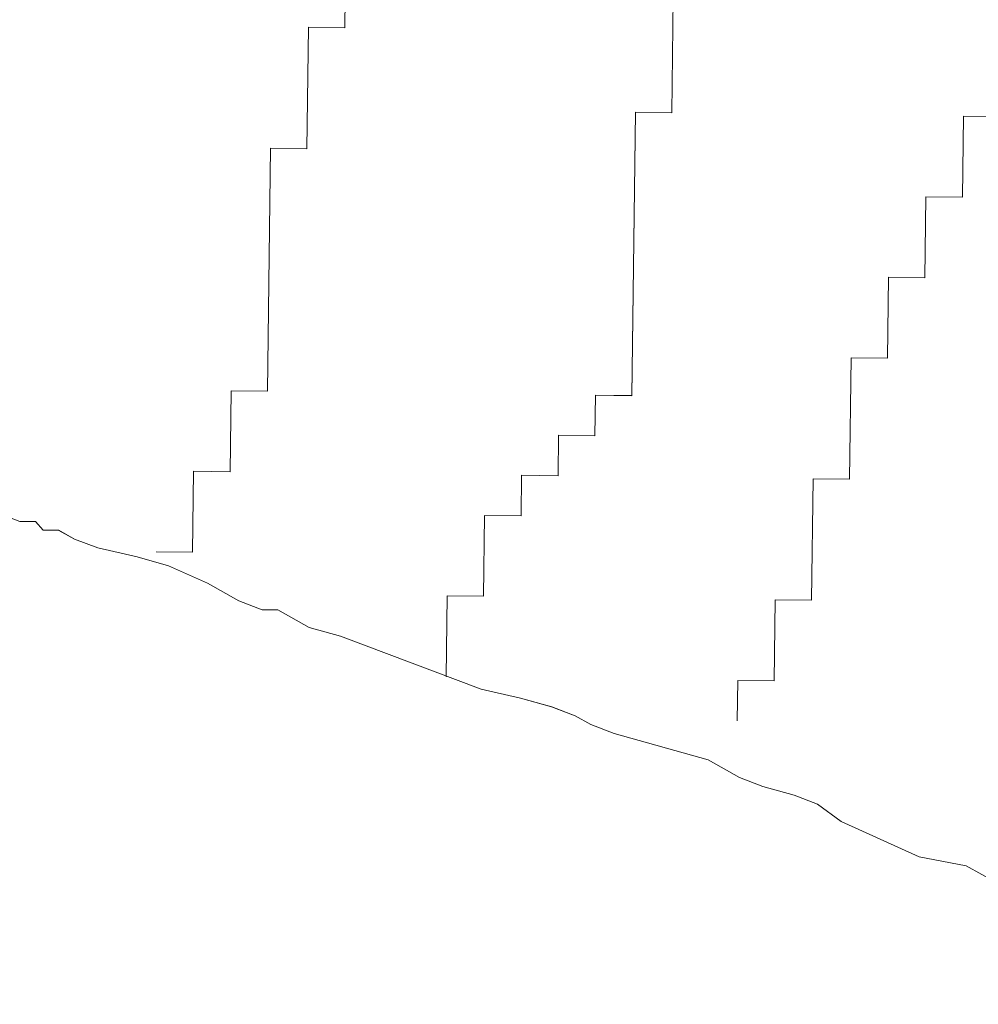
# Model space of a CAD drawing. Units: inches. Extents: x -466983 to 1020, y 324 to 318697.
# Tile 69 of 97: x 647.144 to 650.415, y 939.297 to 942.656. Entities that reach past the tile are written whole.
import ezdxf

# ---------------------------------------------------------------- set-up
doc = ezdxf.new("R2010")
doc.units = ezdxf.units.IN
doc.header["$MEASUREMENT"] = 0
doc.layers.add('A-FLOR-PATT', color=252, linetype='Continuous', lineweight=13)
doc.layers.add('A-FURN', color=8, linetype='Continuous', lineweight=18)

# ---------------------------------------------------------------- blocks, each defined once
blk = doc.blocks.new('L Shaped Sofa')
at = {"ltscale": 2}
for p, q in [((2406.5409, 749.1822), (2406.7354, 749.0728)), ((2406.7354, 749.0728), (2407.0279, 749.0173)), ((2407.0279, 749.0173), (2407.5145, 748.7981)), ((2407.5145, 748.7981), (2407.6602, 748.689)), ((2407.6602, 748.689), (2407.8063, 748.6341)), ((2407.8063, 748.6341), (2408.0011, 748.579)), ((2408.0011, 748.579), (2408.1472, 748.524)), ((2408.1472, 748.524), (2408.3417, 748.4147)), ((2408.3417, 748.4147), (2408.9262, 748.2493)), ((2408.9262, 748.2493), (2409.0723, 748.1944)), ((2408.1572, 747.9198), (2408.1602, 748.1717)), ((2409.0723, 748.1944), (2409.1695, 748.1397)), ((2409.1695, 748.1397), (2409.3156, 748.0848)), ((2409.3156, 748.0848), (2409.5104, 748.0297)), ((2409.5104, 748.0297), (2409.7541, 747.9743)), ((2409.7541, 747.9743), (2410.6304, 747.6449)), ((2407.9242, 747.4188), (2407.9303, 747.9226)), ((2407.9303, 747.9226), (2408.1572, 747.9198)), ((2409.9657, 747.3938), (2409.9719, 747.8976)), ((2410.6304, 747.6449), (2410.8252, 747.5898)), ((2410.8252, 747.5898), (2411.0198, 747.4804)), ((2411.0198, 747.4804), (2411.1173, 747.48)), ((2411.1173, 747.48), (2411.2634, 747.4251)), ((2407.6881, 746.6658), (2407.6973, 747.4215)), ((2407.6973, 747.4215), (2407.9242, 747.4188)), ((2411.2634, 747.4251), (2411.4579, 747.3157)), ((2409.7327, 746.8928), (2409.7389, 747.3966)), ((2409.7389, 747.3966), (2409.9657, 747.3938)), ((2411.4579, 747.3157), (2411.7012, 747.2062)), ((2411.7012, 747.2062), (2411.8961, 747.151)), ((2411.5443, 746.6187), (2411.5505, 747.1225)), ((2411.5505, 747.1225), (2411.7773, 747.1197)), ((2411.8961, 747.151), (2412.1397, 747.0957)), ((2412.1397, 747.0957), (2412.2858, 747.0408)), ((2412.2858, 747.0408), (2412.383, 746.9861)), ((2412.383, 746.9861), (2412.4806, 746.9856)), ((2412.4806, 746.9856), (2412.5291, 746.9312)), ((2412.5291, 746.9312), (2412.6267, 746.9307)), ((2409.5028, 746.6436), (2409.5059, 746.8955)), ((2409.5059, 746.8955), (2409.7327, 746.8928)), ((2407.452, 745.9128), (2407.4613, 746.6686)), ((2407.4613, 746.6686), (2407.6881, 746.6658)), ((2409.2729, 746.3945), (2409.276, 746.6464)), ((2409.276, 746.6464), (2409.5028, 746.6436)), ((2411.3113, 746.1176), (2411.3175, 746.6215)), ((2411.3175, 746.6215), (2411.5443, 746.6187)), ((2409.043, 746.1454), (2409.0461, 746.3973)), ((2409.0461, 746.3973), (2409.2729, 746.3945)), ((2408.7946, 744.3847), (2408.8161, 746.1481)), ((2408.8161, 746.1481), (2409.043, 746.1454)), ((2411.066, 744.6089), (2411.0845, 746.1204)), ((2411.0845, 746.1204), (2411.3113, 746.1176)), ((2407.219, 745.4118), (2407.2252, 745.9156)), ((2407.2252, 745.9156), (2407.452, 745.9128)), ((2406.9861, 744.9107), (2406.9922, 745.4146)), ((2406.9922, 745.4146), (2407.219, 745.4118)), ((2406.7531, 744.4097), (2406.7592, 744.9135)), ((2406.7592, 744.9135), (2406.9861, 744.9107)), ((2410.83, 743.856), (2410.8392, 744.6117)), ((2410.8392, 744.6117), (2411.066, 744.6089)), ((2406.5262, 744.4125), (2406.7531, 744.4097)), ((2408.5493, 742.876), (2408.5678, 744.3875)), ((2408.5678, 744.3875), (2408.7946, 744.3847)), ((2410.597, 743.3549), (2410.6031, 743.8587)), ((2410.6031, 743.8587), (2410.83, 743.856))]:
    blk.add_line(p, q, dxfattribs=at)

msp = doc.modelspace()

# ---------------------------------------------------------------- hatches: boundary and pattern name
at = {"layer": 'A-FLOR-PATT', "transparency": 33554572}
h = msp.add_hatch(dxfattribs=at)
h.set_pattern_fill('ANSI37', color=256, scale=30)
h.set_pattern_definition([(45, (-1212.4137, -290.035), (-2.6516504, 2.6516504), []), (135, (-1212.4137, -290.035), (-2.6516504, -2.6516504), [])])
h.paths.add_polyline_path([(901.8057, 1075.9377), (900.6144, 1075.9377), (900.6144, 1065.3856), (899.391, 1065.3856), (898.0911, 1065.3856), (892.8356, 1058.7098, -0.258377), (892.1875, 1058.3509), (879.9848, 1058.3509, -0.20177), (879.4382, 1058.5808), (874.0812, 1065.3856), (872.7813, 1065.3856), (871.5579, 1065.3856), (871.5579, 1075.9377), (813.8057, 1075.9377), (813.8057, 1044.7922), (832.3947, 1044.7922, -0.394795), (848.6602, 1028.5356), (848.6602, 1009.9377), (901.8057, 1009.9377), (901.8057, 1015.9377), (901.3057, 1015.9377), (871.3057, 1015.9377), (871.3057, 1017.2502), (871.3344, 1017.2502, -0.401453), (901.3057, 1045.9377), (901.8057, 1045.9377)])
edge = h.paths.add_edge_path(flags=16)
edge.add_line((847.7731, 1068.9486), (847.7731, 1073.7088))
edge.add_arc((849.2269, 1073.7088), 1.4538, 90, 180, ccw=False)
edge.add_line((849.2269, 1075.1627), (864.4921, 1075.1627))
edge.add_arc((864.4921, 1073.7088), 1.4538, 0, 90, ccw=False)
edge.add_line((865.9459, 1073.7088), (865.9459, 1069.0035))
edge.add_arc((832.6447, 1068.9761), 33.3012, -20.61234, 0.04725, ccw=False)
edge.add_ellipse((856.8595, 1058.48), major_axis=(0, 10.2131), ratio=0.6859192, start_angle=100.00884, end_angle=259.99116, ccw=False)
edge.add_arc((881.0742, 1068.9761), 33.3012, 180.04725, 200.61234, ccw=False)
h.paths.add_polyline_path([(853.1456, 1066.4815), (853.1456, 1066.4534), (853.1463, 1066.4534, 0.433107), (852.9166, 1066.6849), (852.9166, 1066.4534), (853.1456, 1066.4534), (853.1456, 1066.4815), (853.088, 1066.6122, 0.697939), (852.6995, 1066.4534), (852.7003, 1066.4534), (852.7003, 1066.4815), (852.9166, 1067.0012), (852.9166, 1066.6849, -0.396254)], flags=0)
h.paths.add_polyline_path([(861.0187, 1066.4815), (861.0187, 1066.4534), (861.0194, 1066.4534, 0.416404), (860.8024, 1066.6849), (860.8024, 1066.4534), (861.0187, 1066.4534), (861.0187, 1066.4815), (860.9672, 1066.6053, 0.713344), (860.5726, 1066.4534), (860.5734, 1066.4534), (860.5734, 1066.4815), (860.8024, 1067.0012), (860.8024, 1066.6849, -0.379973)], flags=0)
edge = h.paths.add_edge_path(flags=0)
edge.add_spline(control_points=[(861.1298, 1065.7855), (861.4661, 1065.2478), (861.6134, 1065.0161), (861.9833, 1064.3736), (862.1924, 1063.9443), (862.5614, 1063.0391), (862.7212, 1062.5633), (862.9865, 1061.5781), (863.092, 1061.0689), (863.2452, 1060.031), (863.293, 1059.5025), (863.3295, 1058.4409), (863.3181, 1057.9078), (863.2366, 1056.8518), (863.1664, 1056.3289), (862.9695, 1055.308), (862.8427, 1054.8099), (862.5365, 1053.8522), (862.3571, 1053.3927), (861.9514, 1052.5249), (861.7251, 1052.1166), (861.233, 1051.3622), (860.9672, 1051.0162), (860.4048, 1050.3949), (860.1082, 1050.1197), (859.4937, 1049.6461), (859.1758, 1049.4476), (858.5276, 1049.1299), (858.1973, 1049.0107), (857.5315, 1048.8518), (857.1959, 1048.8121), (856.5249, 1048.812), (856.1894, 1048.8515), (855.5236, 1049.0101), (855.1933, 1049.1291), (854.545, 1049.4465), (854.2271, 1049.6449), (853.6124, 1050.1183), (853.3158, 1050.3933), (852.7533, 1051.0143), (852.4874, 1051.3602), (851.9952, 1052.1144), (851.7688, 1052.5225), (851.3629, 1053.3902), (851.1834, 1053.8496), (850.877, 1054.8071), (850.7501, 1055.3051), (850.553, 1056.326), (850.4827, 1056.8488), (850.401, 1057.9048), (850.3895, 1058.4379), (850.4257, 1059.4995), (850.4734, 1060.0281), (850.6265, 1061.066), (850.7318, 1061.5753), (850.9969, 1062.5605), (851.1567, 1063.0365), (851.5254, 1063.9418), (851.7345, 1064.3712), (852.1056, 1065.0164), (852.2544, 1065.2503), (852.6082, 1065.7335)], knot_values=[3.915332, 3.915332, 3.915332, 3.915332, 4.013468, 4.013468, 4.175532, 4.175532, 4.337596, 4.337596, 4.49966, 4.49966, 4.661724, 4.661724, 4.823788, 4.823788, 4.985852, 4.985852, 5.147916, 5.147916, 5.30998, 5.30998, 5.472044, 5.472044, 5.634109, 5.634109, 5.796173, 5.796173, 5.958237, 5.958237, 6.120301, 6.120301, 6.282365, 6.282365, 6.444429, 6.444429, 6.606493, 6.606493, 6.768557, 6.768557, 6.930621, 6.930621, 7.092685, 7.092685, 7.254749, 7.254749, 7.416813, 7.416813, 7.578878, 7.578878, 7.740942, 7.740942, 7.903006, 7.903006, 8.06507, 8.06507, 8.227134, 8.227134, 8.389198, 8.389198, 8.551262, 8.551262, 8.65037, 8.65037, 8.65037, 8.65037], degree=3, periodic=0)
edge.add_line((852.6421, 1065.7855), (861.1298, 1065.7855))
edge = h.paths.add_edge_path(flags=0)
edge.add_ellipse((856.8496, 1057.7432), major_axis=(0, 7.7921), ratio=0.687861, start_angle=0, end_angle=360)
h.paths.add_polyline_path([(848.8634, 1069.3891), (848.8634, 1073.9605, -0.414214), (849.9538, 1075.0508), (863.7652, 1075.0508, -0.414214), (864.8555, 1073.9605), (864.8555, 1069.3891, -0.388936), (864.5237, 1069.027, -0.043561), (849.1953, 1069.027, -0.388936)], flags=0)
h.paths.add_polyline_path([(853.1006, 1068.1122, -1), (852.6775, 1068.1122, -1)], flags=0)
edge = h.paths.add_edge_path(flags=0)
edge.add_ellipse((856.8595, 1057.3378), major_axis=(0, 2.207), ratio=0.657164, start_angle=0, end_angle=360)
h.paths.add_polyline_path([(861.0415, 1068.1122, -1), (860.6184, 1068.1122, -1)], flags=0)
edge = h.paths.add_edge_path()
edge.add_line((573.9537, 1057.3412), (573.9537, 1075.9377))
edge.add_line((573.9537, 1075.9377), (558.7308, 1075.9377))
edge.add_line((558.7308, 1075.9377), (558.7308, 1065.3856))
edge.add_line((558.7308, 1065.3856), (557.5074, 1065.3856))
edge.add_line((557.5074, 1065.3856), (556.2075, 1065.3856))
edge.add_line((556.2075, 1065.3856), (550.952, 1058.7098))
edge.add_arc((550.3039, 1059.1155), 0.7646, 270, 327.9483, ccw=False)
edge.add_line((550.3039, 1058.3509), (538.1012, 1058.3509))
edge.add_arc((538.1012, 1059.1155), 0.7646, 224.3704, 270, ccw=False)
edge.add_line((537.5546, 1058.5808), (532.1976, 1065.3856))
edge.add_line((532.1976, 1065.3856), (530.8977, 1065.3856))
edge.add_line((530.8977, 1065.3856), (529.6743, 1065.3856))
edge.add_line((529.6743, 1065.3856), (529.6743, 1075.9377))
edge.add_line((529.6743, 1075.9377), (520.8057, 1075.9377))
edge.add_line((520.8057, 1075.9377), (520.8057, 1045.9377))
edge.add_line((520.8057, 1045.9377), (521.3057, 1045.9377))
edge.add_arc((521.3057, 1015.9377), 30, 2.50749, 90, ccw=False)
edge.add_line((551.277, 1017.2502), (551.3057, 1017.2502))
edge.add_line((551.3057, 1017.2502), (551.3057, 1015.9377))
edge.add_line((551.3057, 1015.9377), (520.8057, 1015.9377))
edge.add_line((520.8057, 1015.9377), (520.8057, 1009.9377))
edge.add_line((520.8057, 1009.9377), (559.1913, 1010.4022))
edge.add_arc((559.1913, 1011.856), 1.4538, 180, 270, ccw=False)
edge.add_line((557.7375, 1011.856), (557.7375, 1016.5613))
edge.add_arc((591.0386, 1016.5888), 33.3012, 159.38766, 180.04725, ccw=False)
edge.add_ellipse((566.8239, 1027.0848), major_axis=(0, 10.2131), ratio=0.6859192, start_angle=280.00884, end_angle=439.99116, ccw=False)
edge.add_arc((542.6091, 1016.5888), 33.3012, 0.04725, 20.61234, ccw=False)
edge.add_line((575.9103, 1016.6162), (575.9103, 1011.856))
edge.add_arc((574.4565, 1011.856), 1.4538, -90, 0, ccw=False)
edge.add_line((574.4565, 1010.4022), (608.8057, 1009.9377))
edge.add_line((608.8057, 1009.9377), (608.8057, 1041.0857))
edge.add_line((608.8057, 1041.0857), (590.2179, 1041.0857))
edge.add_arc((590.775, 1057.9074), 16.8309, 181.92775, 268.10321, ccw=False)
edge = h.paths.add_edge_path()
edge.add_ellipse((494.2443, 583.6204), major_axis=(0, 10.2131), ratio=0.6859192, start_angle=280.00884, end_angle=439.99116, ccw=False)
edge.add_arc((470.0296, 573.1243), 33.3012, 0.04725, 20.61234, ccw=False)
edge.add_line((503.3307, 573.1518), (503.3307, 568.3916))
edge.add_arc((501.8769, 568.3916), 1.4538, -90, 0, ccw=False)
edge.add_line((501.8769, 566.9377), (539.8057, 566.9377))
edge.add_line((539.8057, 566.9377), (539.8057, 572.9377))
edge.add_line((539.8057, 572.9377), (539.3057, 572.9377))
edge.add_line((539.3057, 572.9377), (509.3057, 572.9377))
edge.add_line((509.3057, 572.9377), (509.3057, 574.2502))
edge.add_line((509.3057, 574.2502), (509.3344, 574.2502))
edge.add_arc((539.3057, 572.9377), 30, 90, 177.49251, ccw=False)
edge.add_line((539.3057, 602.9377), (539.8057, 602.9377))
edge.add_line((539.8057, 602.9377), (539.8057, 626.9377))
edge.add_line((539.8057, 626.9377), (531.7718, 626.9377))
edge.add_line((531.7718, 626.9377), (531.7718, 616.3856))
edge.add_line((531.7718, 616.3856), (530.5484, 616.3856))
edge.add_line((530.5484, 616.3856), (529.2485, 616.3856))
edge.add_line((529.2485, 616.3856), (523.7105, 609.3509))
edge.add_line((523.7105, 609.3509), (510.7766, 609.3509))
edge.add_line((510.7766, 609.3509), (505.2386, 616.3856))
edge.add_line((505.2386, 616.3856), (503.9387, 616.3856))
edge.add_line((503.9387, 616.3856), (502.7153, 616.3856))
edge.add_line((502.7153, 616.3856), (502.7153, 626.9377))
edge.add_line((502.7153, 626.9377), (481.6983, 626.9377))
edge.add_line((481.6983, 626.9377), (481.6983, 610.995))
edge.add_arc((467.2703, 611.4728), 14.4359, 271.92775, 358.10321, ccw=False)
edge.add_line((467.7559, 597.0451), (451.8057, 597.0451))
edge.add_line((451.8057, 597.0451), (451.8057, 584.4035))
edge.add_line((451.8057, 584.4035), (451.8057, 566.9377))
edge.add_line((451.8057, 566.9377), (486.6117, 566.9377))
edge.add_arc((486.6117, 568.3916), 1.4538, 180, 270, ccw=False)
edge.add_line((485.1579, 568.3916), (485.1579, 573.0969))
edge.add_arc((518.4591, 573.1243), 33.3012, 159.38766, 180.04725, ccw=False)
h.paths.add_polyline_path([(836.2609, 1020.7328), (879.8898, 1020.7328), (879.8898, 1039.3902), (836.2609, 1039.3902)], flags=25)
h.paths.add_polyline_path([(549.9851, 1036.7492), (593.614, 1036.7492), (593.614, 1055.4065), (549.9851, 1055.4065)], flags=24)
h.paths.add_polyline_path([(475.123, 595.5959), (518.752, 595.5959), (518.752, 614.2532), (475.123, 614.2532)], flags=24)
h = msp.add_hatch(dxfattribs=at)
h.set_pattern_fill('ANSI37', color=256, scale=20)
h.set_pattern_definition([(45, (-1212.4137, -290.035), (-1.767767, 1.767767), []), (135, (-1212.4137, -290.035), (-1.767767, -1.767767), [])])
h.paths.add_polyline_path([(809.8057, 870.9377), (809.8057, 888.1519), (806.9985, 888.1519), (802.6624, 888.1519), (789.3832, 888.1519), (786.2846, 888.1519, -0.414214), (785.4991, 888.9374), (785.4991, 900.1959), (785.4991, 908.4696, -0.414214), (786.8082, 909.7787, -0.414214), (785.4991, 911.0878), (785.4991, 929.1015, -0.414214), (786.8082, 930.4106, -0.414214), (785.4991, 931.7197), (785.4991, 931.9039, -0.414214), (784.19, 930.5948), (766.7223, 930.5948, -0.412359), (765.4132, 931.8956, -0.413741), (764.1145, 930.5782), (744.5781, 930.422, -0.416556), (743.7864, 931.2075), (743.7864, 933.5153), (742.2154, 933.5153), (742.2154, 952.024, -0.001344), (743.7864, 952.1998), (743.7864, 953.9377), (678.5915, 953.9377), (678.5915, 951.1305), (678.5915, 946.7945), (678.5915, 933.5153), (678.5915, 930.4166, -0.414214), (677.806, 929.6312), (666.5475, 929.6312), (658.2738, 929.6312, -0.414214), (656.9647, 930.9403, -0.414214), (655.6556, 929.6312), (637.6419, 929.6312, -0.414214), (636.3328, 930.9403, -0.414214), (635.0237, 929.6312), (634.8395, 929.6312, -0.414214), (636.1486, 928.322), (636.1486, 910.8544, -0.412359), (634.8478, 909.5452, -0.413741), (636.1653, 908.2466), (636.3214, 888.7102, -0.416556), (635.5359, 887.9184), (633.2281, 887.9184), (633.2281, 886.3475), (614.7194, 886.3475, -0.001344), (614.5436, 887.9184), (612.8057, 887.9184), (612.8057, 834.9377), (612.8057, 752.9377), (612.8057, 748.9377), (612.8057, 697.9377), (654.8057, 697.9377), (654.8057, 701.9377), (715.8057, 701.9377), (715.8057, 737.4353), (774.2918, 737.4353), (774.2918, 795.9377), (809.8057, 795.9377)])
h.paths.add_polyline_path([(679.2761, 849.5757, 0.102523), (682.1475, 849.2608, -0.080461), (694.5428, 849.7725, -0.283899), (694.4822, 849.0082, 0.136605), (694.4068, 848.8103, -0.030441), (694.5428, 846.8929), (694.5428, 842.6198), (694.5428, 838.3466, -0.028219), (694.4246, 836.5684), (694.425, 836.5684, 0.196187), (694.4456, 836.2708, -0.302897), (694.5428, 835.467, -0.080461), (682.1475, 835.9787, 0.102523), (679.2761, 835.6638, -0.58611), (678.6457, 836.0169), (678.6457, 849.2227, -0.58611)], flags=16)
h.paths.add_polyline_path([(679.5173, 848.6515, 0.699597), (679.476, 848.6342, 1.20716), (679.1935, 848.7422, 0.010621)], flags=0)
h.paths.add_polyline_path([(679.4923, 836.5608, -0.013798), (679.9178, 836.6594, -0.071703), (682.8533, 837.1434, -0.165743), (682.1665, 839.1006), (682.1665, 842.6094), (682.1665, 846.0603, -0.240616), (683.4733, 848.6767, -0.068263), (693.9295, 849.0082), (693.7875, 848.7083), (693.7875, 849.0228, 0.067332), (683.4733, 848.6767, 0.240616), (682.1665, 846.0603), (682.1665, 842.6094), (682.1665, 839.1006, 0.23459), (683.461, 836.5513, 0.068093), (693.7875, 836.1955), (693.7875, 836.5104), (693.9296, 836.2102, -0.077215), (682.2421, 836.7815, 0.086627), (679.5283, 836.5701, -0.628402), (679.5029, 836.5735), (679.5029, 836.6071, 0.910458)], flags=0)
h.paths.add_polyline_path([(679.476, 848.6364), (679.2069, 848.647), (679.2069, 836.5718, 0.913566), (679.3645, 836.5861), (679.476, 836.5824)], flags=0)
h.paths.add_polyline_path([(679.2761, 829.8604, 0.102523), (682.1475, 829.5455, -0.080461), (694.5428, 830.0572, -0.283899), (694.4822, 829.2929, 0.136605), (694.4068, 829.095, -0.030441), (694.5428, 827.1776), (694.5428, 822.9045), (694.5428, 818.6314, -0.028219), (694.4246, 816.8531), (694.425, 816.8532, 0.196187), (694.4456, 816.5555, -0.302897), (694.5428, 815.7517, -0.080461), (682.1475, 816.2635, 0.102523), (679.2761, 815.9485, -0.58611), (678.6457, 816.3016), (678.6457, 829.5074, -0.58611)], flags=16)
h.paths.add_polyline_path([(679.5173, 828.9362, 0.699597), (679.476, 828.9189, 1.20716), (679.1935, 829.0269, 0.010621)], flags=0)
h.paths.add_polyline_path([(679.4923, 816.8456, -0.013798), (679.9178, 816.9441, -0.071703), (682.8533, 817.4281, -0.165743), (682.1665, 819.3853), (682.1665, 822.8941), (682.1665, 826.345, -0.240616), (683.4733, 828.9614, -0.068263), (693.9295, 829.2929), (693.7875, 828.9931), (693.7875, 829.3076, 0.067332), (683.4733, 828.9614, 0.240616), (682.1665, 826.345), (682.1665, 822.8941), (682.1665, 819.3853, 0.23459), (683.461, 816.836, 0.068093), (693.7875, 816.4802), (693.7875, 816.7952), (693.9296, 816.4949, -0.077215), (682.2421, 817.0662, 0.086627), (679.5283, 816.8549, -0.628402), (679.5029, 816.8582), (679.5029, 816.8918, 0.910458)], flags=0)
h.paths.add_polyline_path([(679.476, 828.9211), (679.2069, 828.9317), (679.2069, 816.8565, 0.913566), (679.3645, 816.8708), (679.476, 816.8671)], flags=0)
h.paths.add_polyline_path([(679.2761, 810.1451, 0.102523), (682.1475, 809.8302, -0.080461), (694.5428, 810.342, -0.3023), (694.4466, 809.5394, 0.10023), (694.4058, 809.3878, -0.03057), (694.5428, 807.4623), (694.5428, 803.1892), (694.5428, 798.9161, -0.03057), (694.4058, 796.9906, 0.10023), (694.4466, 796.839, -0.3023), (694.5428, 796.0365, -0.080461), (682.1475, 796.5482, 0.102523), (679.2761, 796.2333, -0.58611), (678.6457, 796.5863), (678.6457, 809.7921, -0.58611)], flags=16)
h.paths.add_polyline_path([(679.5173, 809.2417, 0.699597), (679.476, 809.2244, 1.20716), (679.1935, 809.3324, 0.010621)], flags=0)
h.paths.add_polyline_path([(679.4923, 797.151, -0.013798), (679.9178, 797.2496, -0.071703), (682.8533, 797.7336, -0.165743), (682.1665, 799.6908), (682.1665, 803.1996), (682.1665, 806.6505, -0.239349), (683.461, 809.2577, -0.072465), (694.4468, 809.5405, 0.197932), (694.425, 809.2405), (693.7875, 809.2985), (693.7875, 809.6135, 0.068093), (683.461, 809.2577, 0.239349), (682.1665, 806.6505), (682.1665, 803.1996), (682.1665, 799.6908, 0.235854), (683.4733, 797.1323, 0.067332), (693.7875, 796.7861), (693.7875, 797.1006), (694.425, 797.1586, 0.197932), (694.4468, 796.8586, -0.080419), (682.1557, 797.3795, 0.083867), (679.5283, 797.1603, -0.628402), (679.5029, 797.1637), (679.5029, 797.1973, 0.910458)], flags=0)
h.paths.add_polyline_path([(679.2069, 809.2372), (679.2069, 797.162, 0.913566), (679.3645, 797.1763), (679.476, 797.1726), (679.476, 809.2266)], flags=0)
h.paths.add_polyline_path([(695.3643, 853.2989), (728.2231, 853.2989), (728.2231, 771.1519), (695.3643, 771.1519)], flags=16)
h.paths.add_polyline_path([(696.0215, 852.6417), (727.5659, 852.6417), (727.5659, 771.809), (696.0215, 771.809)], flags=0)
h.paths.add_polyline_path([(679.2761, 788.7869, 0.102523), (682.1475, 788.472, -0.080461), (694.5428, 788.9837, -0.3023), (694.4466, 788.1812, 0.10023), (694.4058, 788.0296, -0.03057), (694.5428, 786.1041), (694.5428, 781.831), (694.5428, 777.5578, -0.03057), (694.4058, 775.6323, 0.10023), (694.4466, 775.4808, -0.3023), (694.5428, 774.6782, -0.080461), (682.1475, 775.19, 0.102523), (679.2761, 774.875, -0.58611), (678.6457, 775.2281), (678.6457, 788.4339, -0.58611)], flags=16)
h.paths.add_polyline_path([(679.5173, 787.8834, 0.699597), (679.476, 787.8662, 1.20716), (679.1935, 787.9742, 0.010621)], flags=0)
h.paths.add_polyline_path([(679.4923, 775.7928, -0.013798), (679.9178, 775.8914, -0.071703), (682.8533, 776.3753, -0.165743), (682.1665, 778.3325), (682.1665, 781.8414), (682.1665, 785.2922, -0.239349), (683.461, 787.8995, -0.072465), (694.4468, 788.1823, 0.197932), (694.425, 787.8823), (693.7875, 787.9403), (693.7875, 788.2553, 0.068093), (683.461, 787.8995, 0.239349), (682.1665, 785.2922), (682.1665, 781.8414), (682.1665, 778.3325, 0.235854), (683.4733, 775.7741, 0.067332), (693.7875, 775.4279), (693.7875, 775.7424), (694.425, 775.8004, 0.197932), (694.4468, 775.5004, -0.080419), (682.1557, 776.0212, 0.083867), (679.5283, 775.8021, -0.628402), (679.5029, 775.8054), (679.5029, 775.8391, 0.910458)], flags=0)
h.paths.add_polyline_path([(679.2069, 787.8789), (679.2069, 775.8038, 0.913566), (679.3645, 775.818), (679.476, 775.8144), (679.476, 787.8684)], flags=0)
h.paths.add_polyline_path([(704.641, 854.1204, -0.080461), (705.1527, 866.5157, 0.102523), (704.8378, 869.3871, -0.58611), (705.1908, 870.0174), (718.3966, 870.0174, -0.58611), (718.7496, 869.3871, 0.102523), (718.4347, 866.5157, -0.080461), (718.9465, 854.1204, -0.3023), (718.1439, 854.2166, 0.10023), (717.9924, 854.2574, -0.03057), (716.0668, 854.1204), (711.7937, 854.1204), (707.5206, 854.1204, -0.03057), (705.5951, 854.2574, 0.10023), (705.4435, 854.2166, -0.3023)], flags=16)
h.paths.add_polyline_path([(717.8462, 869.1459, 0.699597), (717.8289, 869.1872, 1.20716), (717.9369, 869.4697, 0.010621)], flags=0)
h.paths.add_polyline_path([(705.4631, 854.2164, -0.080419), (705.984, 866.5074, 0.083867), (705.7648, 869.1349, -0.628402), (705.7682, 869.1603), (705.8018, 869.1603, 0.910458), (705.7555, 869.1709, -0.013798), (705.8541, 868.7454, -0.071703), (706.3381, 865.8099, -0.165743), (708.2953, 866.4967), (711.8041, 866.4967), (715.255, 866.4967, -0.239349), (717.8622, 865.2022, -0.072465), (718.145, 854.2164, 0.197932), (717.845, 854.2382), (717.903, 854.8757), (718.218, 854.8757, 0.068093), (717.8622, 865.2022, 0.239349), (715.255, 866.4967), (711.8041, 866.4967), (708.2953, 866.4967, 0.235854), (705.7368, 865.1898, 0.067332), (705.3906, 854.8757), (705.7051, 854.8757), (705.7631, 854.2382, 0.197932)], flags=16)
h.paths.add_polyline_path([(705.7665, 869.4563, 0.913566), (705.7808, 869.2987), (705.7771, 869.1872), (717.8311, 869.1872), (717.8417, 869.4563)], flags=0)
h.paths.add_polyline_path([(729.0446, 842.6198), (729.0446, 846.8929, -0.03057), (729.1817, 848.8184, 0.10023), (729.1408, 848.9699, -0.3023), (729.0446, 849.7725, -0.080461), (741.4399, 849.2608, 0.102523), (744.3113, 849.5757, -0.58611), (744.9417, 849.2227), (744.9417, 836.0169, -0.58611), (744.3113, 835.6638, 0.102523), (741.4399, 835.9787, -0.080461), (729.0446, 835.467, -0.3023), (729.1408, 836.2696, 0.10023), (729.1817, 836.4211, -0.03057), (729.0446, 838.3466)], flags=16)
h.paths.add_polyline_path([(744.1115, 836.5846, 1.20716), (744.3939, 836.4766, 0.010621), (744.0701, 836.5673, 0.699597)], flags=0)
h.paths.add_polyline_path([(729.1407, 836.2684, 0.197932), (729.1624, 836.5684), (729.7999, 836.5104), (729.7999, 836.1955, 0.068093), (740.1264, 836.5513, 0.239349), (741.4209, 839.1585), (741.4209, 842.6094), (741.4209, 846.1182, 0.235854), (740.1141, 848.6767, 0.067332), (729.7999, 849.0228), (729.7999, 848.7083), (729.1624, 848.6503, 0.197932), (729.1407, 848.9504, -0.080419), (741.4317, 848.4295, 0.083867), (744.0591, 848.6486, -0.628402), (744.0845, 848.6453), (744.0845, 848.6117, 0.910458), (744.0951, 848.6579, -0.013798), (743.6696, 848.5594, -0.071703), (740.7341, 848.0754, -0.165743), (741.4209, 846.1182), (741.4209, 842.6094), (741.4209, 839.1585, -0.239349), (740.1264, 836.5513, -0.072465)], flags=0)
h.paths.add_polyline_path([(729.0446, 830.0572, -0.080461), (741.4399, 829.5455, 0.102523), (744.3113, 829.8604, -0.58611), (744.9417, 829.5074), (744.9417, 816.3016, -0.58611), (744.3113, 815.9485, 0.102523), (741.4399, 816.2635, -0.080461), (729.0446, 815.7517, -0.3023), (729.1408, 816.5543, 0.10023), (729.1817, 816.7058, -0.03057), (729.0446, 818.6314), (729.0446, 822.9045), (729.0446, 827.1776, -0.03057), (729.1817, 829.1031, 0.10023), (729.1408, 829.2547, -0.3023)], flags=16)
h.paths.add_polyline_path([(744.1115, 816.8693, 1.20716), (744.3939, 816.7613, 0.010621), (744.0701, 816.852, 0.699597)], flags=0)
h.paths.add_polyline_path([(729.1407, 829.2351, -0.080419), (741.4317, 828.7142, 0.083867), (744.0591, 828.9334, -0.628402), (744.0845, 828.93), (744.0845, 828.8964, 0.910458), (744.0951, 828.9427, -0.013798), (743.6696, 828.8441, -0.071703), (740.7341, 828.3601, -0.165743), (741.4209, 826.4029), (741.4209, 822.8941), (741.4209, 819.4432, -0.239349), (740.1264, 816.836, -0.072465), (729.1407, 816.5531, 0.197932), (729.1624, 816.8532), (729.7999, 816.7952), (729.7999, 816.4802, 0.068093), (740.1264, 816.836, 0.239349), (741.4209, 819.4432), (741.4209, 822.8941), (741.4209, 826.4029, 0.235854), (740.1141, 828.9614, 0.067332), (729.7999, 829.3076), (729.7999, 828.9931), (729.1624, 828.9351, 0.197932)], flags=16)
h.paths.add_polyline_path([(729.0446, 810.342, -0.080461), (741.4399, 809.8302, 0.102523), (744.3113, 810.1451, -0.58611), (744.9417, 809.7921), (744.9417, 796.5863, -0.58611), (744.3113, 796.2333, 0.102523), (741.4399, 796.5482, -0.080461), (729.0446, 796.0365, -0.283899), (729.1052, 796.8007, 0.136605), (729.1806, 796.9987, -0.030441), (729.0446, 798.9161), (729.0446, 803.1892), (729.0446, 807.4623, -0.028219), (729.1628, 809.2406), (729.1624, 809.2405, 0.196187), (729.1418, 809.5382, -0.302897)], flags=16)
h.paths.add_polyline_path([(744.1115, 797.1748, 1.20716), (744.3939, 797.0668, 0.010621), (744.0701, 797.1575, 0.699597)], flags=0)
h.paths.add_polyline_path([(741.3453, 809.0275, 0.086627), (744.0591, 809.2388, -0.628402), (744.0845, 809.2355), (744.0845, 809.2019, 0.910458), (744.0951, 809.2481, -0.013798), (743.6696, 809.1496, -0.071703), (740.7341, 808.6656, -0.165743), (741.4209, 806.7084), (741.4209, 803.1996), (741.4209, 799.7487, -0.240616), (740.1141, 797.1323, -0.068263), (729.658, 796.8008), (729.7999, 797.1006), (729.7999, 796.7861, 0.067332), (740.1141, 797.1323, 0.240616), (741.4209, 799.7487), (741.4209, 803.1996), (741.4209, 806.7084, 0.23459), (740.1264, 809.2577, 0.068093), (729.7999, 809.6135), (729.7999, 809.2985), (729.6578, 809.5988, -0.077215)], flags=0)
h.paths.add_polyline_path([(704.641, 770.3304, -0.283899), (705.4053, 770.2697, 0.136605), (705.6032, 770.1944, -0.030441), (707.5206, 770.3304), (711.7937, 770.3304), (716.0668, 770.3304, -0.028219), (717.8451, 770.2122), (717.845, 770.2126, 0.196187), (718.1427, 770.2331, -0.302897), (718.9465, 770.3304, -0.080461), (718.4347, 757.9351, 0.102523), (718.7496, 755.0637, -0.58611), (718.3966, 754.4333), (705.1908, 754.4333, -0.58611), (704.8378, 755.0637, 0.102523), (705.1527, 757.9351, -0.080461)], flags=16)
h.paths.add_polyline_path([(705.762, 755.3048, 0.699597), (705.7793, 755.2635, 1.20716), (705.6713, 754.9811, 0.010621)], flags=0)
h.paths.add_polyline_path([(705.4053, 769.717), (705.7051, 769.5751), (705.3906, 769.5751, 0.067332), (705.7368, 759.2609, 0.240616), (708.3532, 757.954), (711.8041, 757.954), (715.3129, 757.954, 0.23459), (717.8622, 759.2485, 0.068093), (718.218, 769.5751), (717.903, 769.5751), (718.2033, 769.7172, -0.077215), (717.632, 758.0297, 0.086627), (717.8433, 755.3159, -0.628402), (717.84, 755.2904), (717.8064, 755.2904, 0.910458), (717.8526, 755.2799, -0.013798), (717.7541, 755.7053, -0.071703), (717.2701, 758.6409, -0.165743), (715.3129, 757.954), (711.8041, 757.954), (708.3532, 757.954, -0.240616), (705.7368, 759.2609, -0.068263)], flags=0)
h.paths.add_polyline_path([(729.0446, 788.9837, -0.080461), (741.4399, 788.472, 0.102523), (744.3113, 788.7869, -0.58611), (744.9417, 788.4339), (744.9417, 775.2281, -0.58611), (744.3113, 774.875, 0.102523), (741.4399, 775.19, -0.080461), (729.0446, 774.6782, -0.283899), (729.1052, 775.4425, 0.136605), (729.1806, 775.6405, -0.030441), (729.0446, 777.5578), (729.0446, 781.831), (729.0446, 786.1041, -0.028219), (729.1628, 787.8823), (729.1624, 787.8823, 0.196187), (729.1418, 788.1799, -0.302897)], flags=16)
h.paths.add_polyline_path([(744.1115, 775.8165, 1.20716), (744.3939, 775.7086, 0.010621), (744.0701, 775.7993, 0.699597)], flags=0)
h.paths.add_polyline_path([(741.3453, 787.6692, 0.086627), (744.0591, 787.8806, -0.628402), (744.0845, 787.8773), (744.0845, 787.8437, 0.910458), (744.0951, 787.8899, -0.013798), (743.6696, 787.7913, -0.071703), (740.7341, 787.3074, -0.165743), (741.4209, 785.3502), (741.4209, 781.8414), (741.4209, 778.3905, -0.240616), (740.1141, 775.7741, -0.068263), (729.658, 775.4425), (729.7999, 775.7424), (729.7999, 775.4279, 0.067332), (740.1141, 775.7741, 0.240616), (741.4209, 778.3905), (741.4209, 781.8414), (741.4209, 785.3502, 0.23459), (740.1264, 787.8995, 0.068093), (729.7999, 788.2553), (729.7999, 787.9403), (729.6578, 788.2405, -0.077215)], flags=0)
h.paths.add_polyline_path([(744.1115, 848.6364), (744.1115, 836.5824), (744.3805, 836.5718), (744.3805, 848.647, 0.913566), (744.2229, 848.6327)], flags=0)
h.paths.add_polyline_path([(744.2229, 828.9174), (744.1115, 828.9211), (744.1115, 816.8671), (744.3805, 816.8565), (744.3805, 828.9317, 0.913566)], flags=0)
h.paths.add_polyline_path([(717.8311, 755.2635), (705.7771, 755.2635), (705.7665, 754.9945), (717.8417, 754.9945, 0.913566), (717.8274, 755.1521)], flags=0)
h.paths.add_polyline_path([(744.2229, 809.2229), (744.1115, 809.2266), (744.1115, 797.1726), (744.3805, 797.162), (744.3805, 809.2372, 0.913566)], flags=0)
h.paths.add_polyline_path([(744.1115, 787.8684), (744.1115, 775.8144), (744.3805, 775.8038), (744.3805, 787.8789, 0.913566), (744.2229, 787.8647)], flags=0)
h.paths.add_polyline_path([(678.8774, 877.1228), (737.6127, 877.1228), (737.6127, 899.5116), (678.8774, 899.5116)], flags=24)

# ---------------------------------------------------------------- linework, layer by layer
at = {"layer": 'A-FURN', "ltscale": 2}
for p, q in [((649.3791, 943.1671), (649.3689, 942.3385)), ((649.3791, 943.1671), (649.3689, 942.3385)), ((649.3791, 943.1671), (649.3689, 942.3385)), ((649.3791, 943.1671), (649.3689, 942.3385)), ((649.3791, 943.1671), (649.3689, 942.3385)), ((649.3791, 943.1671), (649.3689, 942.3385)), ((648.2565, 942.9046), (648.2531, 942.6284)), ((648.2565, 942.9046), (648.2531, 942.6284)), ((648.2565, 942.9046), (648.2531, 942.6284)), ((648.2565, 942.9046), (648.2531, 942.6284)), ((648.2565, 942.9046), (648.2531, 942.6284)), ((648.2565, 942.9046), (648.2531, 942.6284)), ((648.1288, 942.6299), (648.1237, 942.2156)), ((648.1288, 942.6299), (648.1237, 942.2156)), ((648.1288, 942.6299), (648.1237, 942.2156)), ((648.1288, 942.6299), (648.1237, 942.2156)), ((648.1288, 942.6299), (648.1237, 942.2156)), ((648.1288, 942.6299), (648.1237, 942.2156)), ((648.2531, 942.6284), (648.1288, 942.6299)), ((648.2531, 942.6284), (648.1288, 942.6299)), ((648.2531, 942.6284), (648.1288, 942.6299)), ((648.2531, 942.6284), (648.1288, 942.6299)), ((648.2531, 942.6284), (648.1288, 942.6299)), ((648.2531, 942.6284), (648.1288, 942.6299)), ((649.2446, 942.3401), (649.2328, 941.3733)), ((649.2446, 942.3401), (649.2328, 941.3733)), ((649.2446, 942.3401), (649.2328, 941.3733)), ((649.2446, 942.3401), (649.2328, 941.3733)), ((649.2446, 942.3401), (649.2328, 941.3733)), ((649.2446, 942.3401), (649.2328, 941.3733)), ((649.3689, 942.3385), (649.2446, 942.3401)), ((649.3689, 942.3385), (649.2446, 942.3401)), ((649.3689, 942.3385), (649.2446, 942.3401)), ((649.3689, 942.3385), (649.2446, 942.3401)), ((649.3689, 942.3385), (649.2446, 942.3401)), ((649.3689, 942.3385), (649.2446, 942.3401)), ((650.3638, 942.3264), (650.3604, 942.0502)), ((650.3638, 942.3264), (650.3604, 942.0502)), ((650.3638, 942.3264), (650.3604, 942.0502)), ((650.3638, 942.3264), (650.3604, 942.0502)), ((650.3638, 942.3264), (650.3604, 942.0502)), ((650.3638, 942.3264), (650.3604, 942.0502)), ((650.4881, 942.3249), (650.3638, 942.3264)), ((650.4881, 942.3249), (650.3638, 942.3264)), ((650.4881, 942.3249), (650.3638, 942.3264)), ((650.4881, 942.3249), (650.3638, 942.3264)), ((650.4881, 942.3249), (650.3638, 942.3264)), ((650.4881, 942.3249), (650.3638, 942.3264)), ((647.9993, 942.2171), (647.9892, 941.3885)), ((647.9993, 942.2171), (647.9892, 941.3885)), ((647.9993, 942.2171), (647.9892, 941.3885)), ((647.9993, 942.2171), (647.9892, 941.3885)), ((647.9993, 942.2171), (647.9892, 941.3885)), ((647.9993, 942.2171), (647.9892, 941.3885)), ((648.1237, 942.2156), (647.9993, 942.2171)), ((648.1237, 942.2156), (647.9993, 942.2171)), ((648.1237, 942.2156), (647.9993, 942.2171)), ((648.1237, 942.2156), (647.9993, 942.2171)), ((648.1237, 942.2156), (647.9993, 942.2171)), ((648.1237, 942.2156), (647.9993, 942.2171)), ((650.236, 942.0517), (650.2327, 941.7755)), ((650.236, 942.0517), (650.2327, 941.7755)), ((650.236, 942.0517), (650.2327, 941.7755)), ((650.236, 942.0517), (650.2327, 941.7755)), ((650.236, 942.0517), (650.2327, 941.7755)), ((650.236, 942.0517), (650.2327, 941.7755)), ((650.3604, 942.0502), (650.236, 942.0517)), ((650.3604, 942.0502), (650.236, 942.0517)), ((650.3604, 942.0502), (650.236, 942.0517)), ((650.3604, 942.0502), (650.236, 942.0517)), ((650.3604, 942.0502), (650.236, 942.0517)), ((650.3604, 942.0502), (650.236, 942.0517)), ((650.1083, 941.777), (650.1049, 941.5008)), ((650.1083, 941.777), (650.1049, 941.5008)), ((650.1083, 941.777), (650.1049, 941.5008)), ((650.1083, 941.777), (650.1049, 941.5008)), ((650.1083, 941.777), (650.1049, 941.5008)), ((650.1083, 941.777), (650.1049, 941.5008)), ((650.2327, 941.7755), (650.1083, 941.777)), ((650.2327, 941.7755), (650.1083, 941.777)), ((650.2327, 941.7755), (650.1083, 941.777)), ((650.2327, 941.7755), (650.1083, 941.777)), ((650.2327, 941.7755), (650.1083, 941.777)), ((650.2327, 941.7755), (650.1083, 941.777)), ((649.9806, 941.5023), (649.9755, 941.088)), ((649.9806, 941.5023), (649.9755, 941.088)), ((649.9806, 941.5023), (649.9755, 941.088)), ((649.9806, 941.5023), (649.9755, 941.088)), ((649.9806, 941.5023), (649.9755, 941.088)), ((649.9806, 941.5023), (649.9755, 941.088)), ((650.1049, 941.5008), (649.9806, 941.5023)), ((650.1049, 941.5008), (649.9806, 941.5023)), ((650.1049, 941.5008), (649.9806, 941.5023)), ((650.1049, 941.5008), (649.9806, 941.5023)), ((650.1049, 941.5008), (649.9806, 941.5023)), ((650.1049, 941.5008), (649.9806, 941.5023)), ((647.8649, 941.3901), (647.8615, 941.1139)), ((647.8649, 941.3901), (647.8615, 941.1139)), ((647.8649, 941.3901), (647.8615, 941.1139)), ((647.8649, 941.3901), (647.8615, 941.1139)), ((647.8649, 941.3901), (647.8615, 941.1139)), ((647.8649, 941.3901), (647.8615, 941.1139)), ((647.9892, 941.3885), (647.8649, 941.3901)), ((647.9892, 941.3885), (647.8649, 941.3901)), ((647.9892, 941.3885), (647.8649, 941.3901)), ((647.9892, 941.3885), (647.8649, 941.3901)), ((647.9892, 941.3885), (647.8649, 941.3901)), ((647.9892, 941.3885), (647.8649, 941.3901)), ((649.1084, 941.3749), (649.1067, 941.2368)), ((649.1084, 941.3749), (649.1067, 941.2368)), ((649.1084, 941.3749), (649.1067, 941.2368)), ((649.1084, 941.3749), (649.1067, 941.2368)), ((649.1084, 941.3749), (649.1067, 941.2368)), ((649.1084, 941.3749), (649.1067, 941.2368)), ((649.2328, 941.3733), (649.1084, 941.3749)), ((649.2328, 941.3733), (649.1084, 941.3749)), ((649.2328, 941.3733), (649.1084, 941.3749)), ((649.2328, 941.3733), (649.1084, 941.3749)), ((649.2328, 941.3733), (649.1084, 941.3749)), ((649.2328, 941.3733), (649.1084, 941.3749)), ((648.9824, 941.2383), (648.9807, 941.1002)), ((648.9824, 941.2383), (648.9807, 941.1002)), ((648.9824, 941.2383), (648.9807, 941.1002)), ((648.9824, 941.2383), (648.9807, 941.1002)), ((648.9824, 941.2383), (648.9807, 941.1002)), ((648.9824, 941.2383), (648.9807, 941.1002)), ((649.1067, 941.2368), (648.9824, 941.2383)), ((649.1067, 941.2368), (648.9824, 941.2383)), ((649.1067, 941.2368), (648.9824, 941.2383)), ((649.1067, 941.2368), (648.9824, 941.2383)), ((649.1067, 941.2368), (648.9824, 941.2383)), ((649.1067, 941.2368), (648.9824, 941.2383)), ((647.7371, 941.1154), (647.7338, 940.8392)), ((647.7371, 941.1154), (647.7338, 940.8392)), ((647.7371, 941.1154), (647.7338, 940.8392)), ((647.7371, 941.1154), (647.7338, 940.8392)), ((647.7371, 941.1154), (647.7338, 940.8392)), ((647.7371, 941.1154), (647.7338, 940.8392)), ((647.8615, 941.1139), (647.7371, 941.1154)), ((647.8615, 941.1139), (647.7371, 941.1154)), ((647.8615, 941.1139), (647.7371, 941.1154)), ((647.8615, 941.1139), (647.7371, 941.1154)), ((647.8615, 941.1139), (647.7371, 941.1154)), ((647.8615, 941.1139), (647.7371, 941.1154)), ((648.8563, 941.1017), (648.8546, 940.9636)), ((648.8563, 941.1017), (648.8546, 940.9636)), ((648.8563, 941.1017), (648.8546, 940.9636)), ((648.8563, 941.1017), (648.8546, 940.9636)), ((648.8563, 941.1017), (648.8546, 940.9636)), ((648.8563, 941.1017), (648.8546, 940.9636)), ((648.9807, 941.1002), (648.8563, 941.1017)), ((648.9807, 941.1002), (648.8563, 941.1017)), ((648.9807, 941.1002), (648.8563, 941.1017)), ((648.9807, 941.1002), (648.8563, 941.1017)), ((648.9807, 941.1002), (648.8563, 941.1017)), ((648.9807, 941.1002), (648.8563, 941.1017)), ((649.8512, 941.0895), (649.8461, 940.6752)), ((649.8512, 941.0895), (649.8461, 940.6752)), ((649.8512, 941.0895), (649.8461, 940.6752)), ((649.8512, 941.0895), (649.8461, 940.6752)), ((649.8512, 941.0895), (649.8461, 940.6752)), ((649.8512, 941.0895), (649.8461, 940.6752)), ((649.9755, 941.088), (649.8512, 941.0895)), ((649.9755, 941.088), (649.8512, 941.0895)), ((649.9755, 941.088), (649.8512, 941.0895)), ((649.9755, 941.088), (649.8512, 941.0895)), ((649.9755, 941.088), (649.8512, 941.0895)), ((649.9755, 941.088), (649.8512, 941.0895)), ((647.1438, 940.9443), (647.0637, 940.9744)), ((647.1438, 940.9443), (647.0637, 940.9744)), ((647.1438, 940.9443), (647.0637, 940.9744)), ((647.1438, 940.9443), (647.0637, 940.9744)), ((647.1438, 940.9443), (647.0637, 940.9744)), ((647.1438, 940.9443), (647.0637, 940.9744)), ((648.7303, 940.9651), (648.7269, 940.6889)), ((648.7303, 940.9651), (648.7269, 940.6889)), ((648.7303, 940.9651), (648.7269, 940.6889)), ((648.7303, 940.9651), (648.7269, 940.6889)), ((648.7303, 940.9651), (648.7269, 940.6889)), ((648.7303, 940.9651), (648.7269, 940.6889)), ((648.8546, 940.9636), (648.7303, 940.9651)), ((648.8546, 940.9636), (648.7303, 940.9651)), ((648.8546, 940.9636), (648.7303, 940.9651)), ((648.8546, 940.9636), (648.7303, 940.9651)), ((648.8546, 940.9636), (648.7303, 940.9651)), ((648.8546, 940.9636), (648.7303, 940.9651)), ((647.1973, 940.9441), (647.1438, 940.9443)), ((647.1973, 940.9441), (647.1438, 940.9443)), ((647.1973, 940.9441), (647.1438, 940.9443)), ((647.1973, 940.9441), (647.1438, 940.9443)), ((647.1973, 940.9441), (647.1438, 940.9443)), ((647.1973, 940.9441), (647.1438, 940.9443)), ((647.2238, 940.9142), (647.1973, 940.9441)), ((647.2238, 940.9142), (647.1973, 940.9441)), ((647.2238, 940.9142), (647.1973, 940.9441)), ((647.2238, 940.9142), (647.1973, 940.9441)), ((647.2238, 940.9142), (647.1973, 940.9441)), ((647.2238, 940.9142), (647.1973, 940.9441)), ((647.2773, 940.914), (647.2238, 940.9142)), ((647.2773, 940.914), (647.2238, 940.9142)), ((647.2773, 940.914), (647.2238, 940.9142)), ((647.2773, 940.914), (647.2238, 940.9142)), ((647.2773, 940.914), (647.2238, 940.9142)), ((647.2773, 940.914), (647.2238, 940.9142)), ((647.3307, 940.884), (647.2773, 940.914)), ((647.3307, 940.884), (647.2773, 940.914)), ((647.3307, 940.884), (647.2773, 940.914)), ((647.3307, 940.884), (647.2773, 940.914)), ((647.3307, 940.884), (647.2773, 940.914)), ((647.3307, 940.884), (647.2773, 940.914)), ((647.4107, 940.8539), (647.3307, 940.884)), ((647.4107, 940.8539), (647.3307, 940.884)), ((647.4107, 940.8539), (647.3307, 940.884)), ((647.4107, 940.8539), (647.3307, 940.884)), ((647.4107, 940.8539), (647.3307, 940.884)), ((647.4107, 940.8539), (647.3307, 940.884)), ((647.5443, 940.8235), (647.4107, 940.8539)), ((647.5443, 940.8235), (647.4107, 940.8539)), ((647.5443, 940.8235), (647.4107, 940.8539)), ((647.5443, 940.8235), (647.4107, 940.8539)), ((647.5443, 940.8235), (647.4107, 940.8539)), ((647.5443, 940.8235), (647.4107, 940.8539)), ((647.7338, 940.8392), (647.6094, 940.8407)), ((647.7338, 940.8392), (647.6094, 940.8407)), ((647.7338, 940.8392), (647.6094, 940.8407)), ((647.7338, 940.8392), (647.6094, 940.8407)), ((647.7338, 940.8392), (647.6094, 940.8407)), ((647.7338, 940.8392), (647.6094, 940.8407)), ((647.6511, 940.7933), (647.5443, 940.8235)), ((647.6511, 940.7933), (647.5443, 940.8235)), ((647.6511, 940.7933), (647.5443, 940.8235)), ((647.6511, 940.7933), (647.5443, 940.8235)), ((647.6511, 940.7933), (647.5443, 940.8235)), ((647.6511, 940.7933), (647.5443, 940.8235)), ((647.7845, 940.7332), (647.6511, 940.7933)), ((647.7845, 940.7332), (647.6511, 940.7933)), ((647.7845, 940.7332), (647.6511, 940.7933)), ((647.7845, 940.7332), (647.6511, 940.7933)), ((647.7845, 940.7332), (647.6511, 940.7933)), ((647.7845, 940.7332), (647.6511, 940.7933)), ((647.8911, 940.6733), (647.7845, 940.7332)), ((647.8911, 940.6733), (647.7845, 940.7332)), ((647.8911, 940.6733), (647.7845, 940.7332)), ((647.8911, 940.6733), (647.7845, 940.7332)), ((647.8911, 940.6733), (647.7845, 940.7332)), ((647.8911, 940.6733), (647.7845, 940.7332)), ((647.9712, 940.6432), (647.8911, 940.6733)), ((647.9712, 940.6432), (647.8911, 940.6733)), ((647.9712, 940.6432), (647.8911, 940.6733)), ((647.9712, 940.6432), (647.8911, 940.6733)), ((647.9712, 940.6432), (647.8911, 940.6733)), ((647.9712, 940.6432), (647.8911, 940.6733)), ((648.6026, 940.6904), (648.5992, 940.4142)), ((648.6026, 940.6904), (648.5992, 940.4142)), ((648.6026, 940.6904), (648.5992, 940.4142)), ((648.6026, 940.6904), (648.5992, 940.4142)), ((648.6026, 940.6904), (648.5992, 940.4142)), ((648.6026, 940.6904), (648.5992, 940.4142)), ((648.7269, 940.6889), (648.6026, 940.6904)), ((648.7269, 940.6889), (648.6026, 940.6904)), ((648.7269, 940.6889), (648.6026, 940.6904)), ((648.7269, 940.6889), (648.6026, 940.6904)), ((648.7269, 940.6889), (648.6026, 940.6904)), ((648.7269, 940.6889), (648.6026, 940.6904)), ((649.7217, 940.6768), (649.7184, 940.4006)), ((649.7217, 940.6768), (649.7184, 940.4006)), ((649.7217, 940.6768), (649.7184, 940.4006)), ((649.7217, 940.6768), (649.7184, 940.4006)), ((649.7217, 940.6768), (649.7184, 940.4006)), ((649.7217, 940.6768), (649.7184, 940.4006)), ((649.8461, 940.6752), (649.7217, 940.6768)), ((649.8461, 940.6752), (649.7217, 940.6768)), ((649.8461, 940.6752), (649.7217, 940.6768)), ((649.8461, 940.6752), (649.7217, 940.6768)), ((649.8461, 940.6752), (649.7217, 940.6768)), ((649.8461, 940.6752), (649.7217, 940.6768)), ((648.0247, 940.6429), (647.9712, 940.6432)), ((648.0247, 940.6429), (647.9712, 940.6432)), ((648.0247, 940.6429), (647.9712, 940.6432)), ((648.0247, 940.6429), (647.9712, 940.6432)), ((648.0247, 940.6429), (647.9712, 940.6432)), ((648.0247, 940.6429), (647.9712, 940.6432)), ((648.1313, 940.583), (648.0247, 940.6429)), ((648.1313, 940.583), (648.0247, 940.6429)), ((648.1313, 940.583), (648.0247, 940.6429)), ((648.1313, 940.583), (648.0247, 940.6429)), ((648.1313, 940.583), (648.0247, 940.6429)), ((648.1313, 940.583), (648.0247, 940.6429)), ((648.2382, 940.5528), (648.1313, 940.583)), ((648.2382, 940.5528), (648.1313, 940.583)), ((648.2382, 940.5528), (648.1313, 940.583)), ((648.2382, 940.5528), (648.1313, 940.583)), ((648.2382, 940.5528), (648.1313, 940.583)), ((648.2382, 940.5528), (648.1313, 940.583)), ((648.7186, 940.3722), (648.2382, 940.5528)), ((648.7186, 940.3722), (648.2382, 940.5528)), ((648.7186, 940.3722), (648.2382, 940.5528)), ((648.7186, 940.3722), (648.2382, 940.5528)), ((648.7186, 940.3722), (648.2382, 940.5528)), ((648.7186, 940.3722), (648.2382, 940.5528)), ((649.594, 940.4021), (649.5923, 940.264)), ((649.594, 940.4021), (649.5923, 940.264)), ((649.594, 940.4021), (649.5923, 940.264)), ((649.594, 940.4021), (649.5923, 940.264)), ((649.594, 940.4021), (649.5923, 940.264)), ((649.594, 940.4021), (649.5923, 940.264)), ((649.7184, 940.4006), (649.594, 940.4021)), ((649.7184, 940.4006), (649.594, 940.4021)), ((649.7184, 940.4006), (649.594, 940.4021)), ((649.7184, 940.4006), (649.594, 940.4021)), ((649.7184, 940.4006), (649.594, 940.4021)), ((649.7184, 940.4006), (649.594, 940.4021)), ((648.8521, 940.3418), (648.7186, 940.3722)), ((648.8521, 940.3418), (648.7186, 940.3722)), ((648.8521, 940.3418), (648.7186, 940.3722)), ((648.8521, 940.3418), (648.7186, 940.3722)), ((648.8521, 940.3418), (648.7186, 940.3722)), ((648.8521, 940.3418), (648.7186, 940.3722)), ((648.959, 940.3116), (648.8521, 940.3418)), ((648.959, 940.3116), (648.8521, 940.3418)), ((648.959, 940.3116), (648.8521, 940.3418)), ((648.959, 940.3116), (648.8521, 940.3418)), ((648.959, 940.3116), (648.8521, 940.3418)), ((648.959, 940.3116), (648.8521, 940.3418)), ((649.039, 940.2815), (648.959, 940.3116)), ((649.039, 940.2815), (648.959, 940.3116)), ((649.039, 940.2815), (648.959, 940.3116)), ((649.039, 940.2815), (648.959, 940.3116)), ((649.039, 940.2815), (648.959, 940.3116)), ((649.039, 940.2815), (648.959, 940.3116)), ((649.0923, 940.2515), (649.039, 940.2815)), ((649.0923, 940.2515), (649.039, 940.2815)), ((649.0923, 940.2515), (649.039, 940.2815)), ((649.0923, 940.2515), (649.039, 940.2815)), ((649.0923, 940.2515), (649.039, 940.2815)), ((649.0923, 940.2515), (649.039, 940.2815)), ((649.1724, 940.2214), (649.0923, 940.2515)), ((649.1724, 940.2214), (649.0923, 940.2515)), ((649.1724, 940.2214), (649.0923, 940.2515)), ((649.1724, 940.2214), (649.0923, 940.2515)), ((649.1724, 940.2214), (649.0923, 940.2515)), ((649.1724, 940.2214), (649.0923, 940.2515)), ((649.4929, 940.1308), (649.1724, 940.2214)), ((649.4929, 940.1308), (649.1724, 940.2214)), ((649.4929, 940.1308), (649.1724, 940.2214)), ((649.4929, 940.1308), (649.1724, 940.2214)), ((649.4929, 940.1308), (649.1724, 940.2214)), ((649.4929, 940.1308), (649.1724, 940.2214)), ((649.5995, 940.0708), (649.4929, 940.1308)), ((649.5995, 940.0708), (649.4929, 940.1308)), ((649.5995, 940.0708), (649.4929, 940.1308)), ((649.5995, 940.0708), (649.4929, 940.1308)), ((649.5995, 940.0708), (649.4929, 940.1308)), ((649.5995, 940.0708), (649.4929, 940.1308)), ((649.6796, 940.0407), (649.5995, 940.0708)), ((649.6796, 940.0407), (649.5995, 940.0708)), ((649.6796, 940.0407), (649.5995, 940.0708)), ((649.6796, 940.0407), (649.5995, 940.0708)), ((649.6796, 940.0407), (649.5995, 940.0708)), ((649.6796, 940.0407), (649.5995, 940.0708)), ((649.7864, 940.0105), (649.6796, 940.0407)), ((649.7864, 940.0105), (649.6796, 940.0407)), ((649.7864, 940.0105), (649.6796, 940.0407)), ((649.7864, 940.0105), (649.6796, 940.0407)), ((649.7864, 940.0105), (649.6796, 940.0407)), ((649.7864, 940.0105), (649.6796, 940.0407)), ((649.8665, 939.9804), (649.7864, 940.0105)), ((649.8665, 939.9804), (649.7864, 940.0105)), ((649.8665, 939.9804), (649.7864, 940.0105)), ((649.8665, 939.9804), (649.7864, 940.0105)), ((649.8665, 939.9804), (649.7864, 940.0105)), ((649.8665, 939.9804), (649.7864, 940.0105)), ((649.9464, 939.9206), (649.8665, 939.9804)), ((649.9464, 939.9206), (649.8665, 939.9804)), ((649.9464, 939.9206), (649.8665, 939.9804)), ((649.9464, 939.9206), (649.8665, 939.9804)), ((649.9464, 939.9206), (649.8665, 939.9804)), ((649.9464, 939.9206), (649.8665, 939.9804)), ((650.2131, 939.8004), (649.9464, 939.9206)), ((650.2131, 939.8004), (649.9464, 939.9206)), ((650.2131, 939.8004), (649.9464, 939.9206)), ((650.2131, 939.8004), (649.9464, 939.9206)), ((650.2131, 939.8004), (649.9464, 939.9206)), ((650.2131, 939.8004), (649.9464, 939.9206)), ((650.3734, 939.77), (650.2131, 939.8004)), ((650.3734, 939.77), (650.2131, 939.8004)), ((650.3734, 939.77), (650.2131, 939.8004)), ((650.3734, 939.77), (650.2131, 939.8004)), ((650.3734, 939.77), (650.2131, 939.8004)), ((650.3734, 939.77), (650.2131, 939.8004)), ((650.4801, 939.71), (650.3734, 939.77)), ((650.4801, 939.71), (650.3734, 939.77)), ((650.4801, 939.71), (650.3734, 939.77)), ((650.4801, 939.71), (650.3734, 939.77)), ((650.4801, 939.71), (650.3734, 939.77)), ((650.4801, 939.71), (650.3734, 939.77))]:
    msp.add_line(p, q, dxfattribs=at)

# ---------------------------------------------------------------- block references
at = {"layer": 'A-FURN', "xscale": 0.5482153745360612, "yscale": 0.5482153745360612, "zscale": 0.5482153745360612, "rotation": 180}
msp.add_blockref('L Shaped Sofa', (1969.7828, 1350.4232), dxfattribs=at)

doc.saveas('drawing.dxf')
